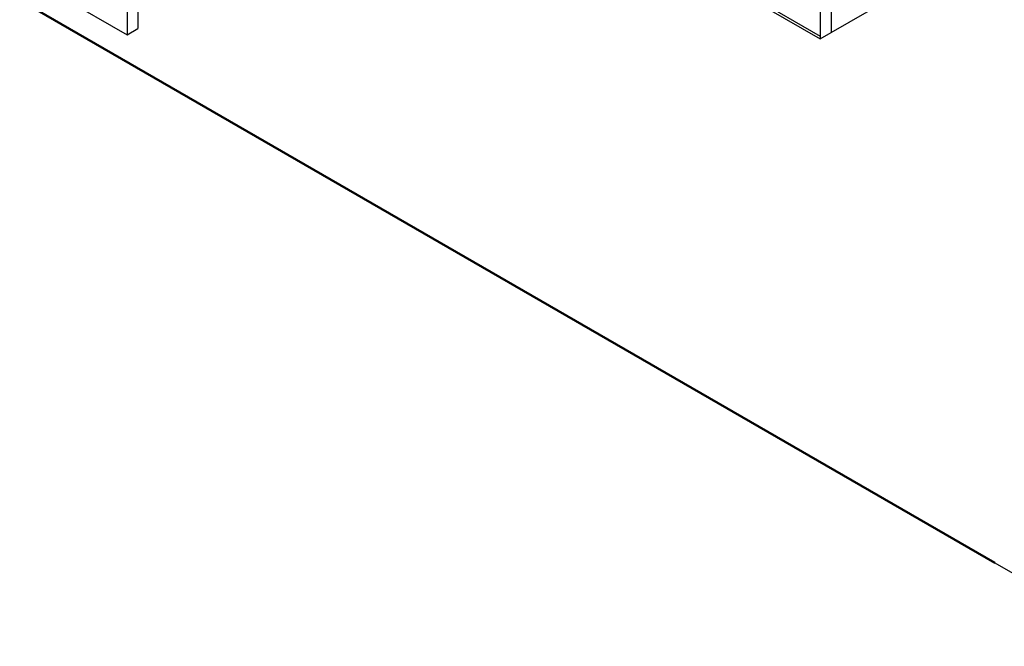
# Model space of a CAD drawing. Units: centimetres. Extents: x 5383 to 11288, y 5305 to 11515.
# Tile 1 of 5: x 5387 to 5675, y 5305 to 5488. Entities that reach past the tile are written whole.
import ezdxf

# ---------------------------------------------------------------- set-up
doc = ezdxf.new("R2010")
doc.units = ezdxf.units.CM
doc.layers.add('A-FLOR-CASE', color=3, linetype='Continuous', lineweight=25)
doc.layers.add('A-WALL', color=7, linetype='Continuous', lineweight=50)

msp = doc.modelspace()

# ---------------------------------------------------------------- linework, layer by layer
at = {"layer": 'A-FLOR-CASE'}
for p, q in [((5421.66, 5639.1), (5421.66, 5485.47)), ((5620.89, 5528.33), (5620.89, 5482.46)), ((5624.1, 5525.39), (5624.1, 5484.31)), ((5555.55, 5520.18), (5620.89, 5482.46)), ((5587.53, 5502.54), (5620.89, 5483.29)), ((5396.53, 5496.36), (5418.53, 5483.66)), ((5418.53, 5492.61), (5418.53, 5483.66)), ((5624.1, 5484.31), (5640.52, 5493.8)), ((5418.53, 5483.66), (5421.66, 5485.47)), ((5620.89, 5482.46), (5624.1, 5484.31)), ((5671.93, 5329.42), (5714.19, 5305.03))]:
    msp.add_line(p, q, dxfattribs=at)
at = {"layer": 'A-WALL'}
msp.add_line((5387.16, 5493.83), (5671.93, 5329.42), dxfattribs=at)

doc.saveas('drawing.dxf')
